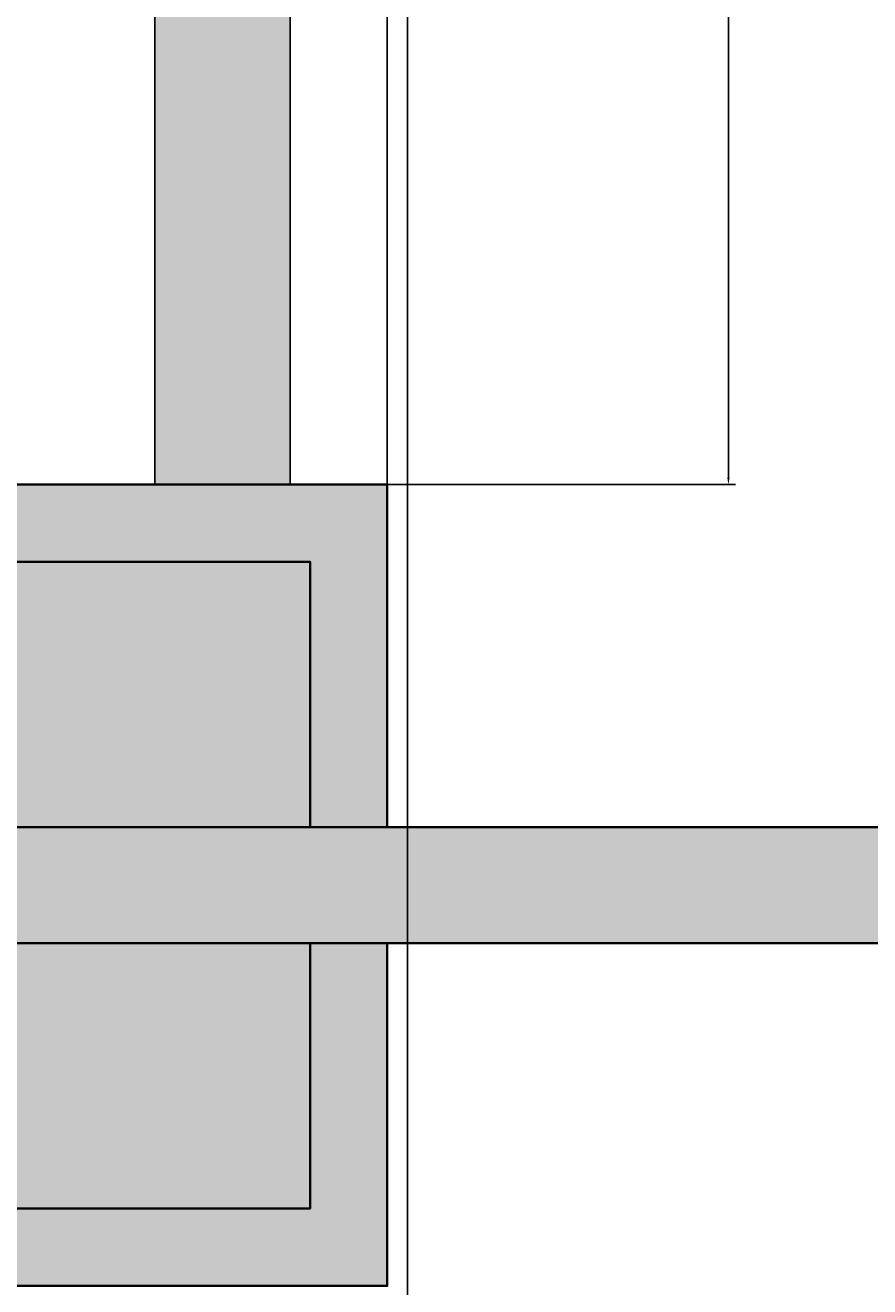
# Model space of a CAD drawing. Units: millimetres. Extents: x -11 to 280, y -4 to 208.
# Tile 36 of 55: x 222 to 244, y 23 to 55. Entities that reach past the tile are written whole.
import ezdxf

# ---------------------------------------------------------------- set-up
doc = ezdxf.new("R2010")
doc.units = ezdxf.units.MM
for name, color, linetype, lineweight in [('M-DIMS', 2, 'Continuous', 18), ('M-HYDR-CYL', 7, 'Continuous', 35), ('M-HYDR-CYL-PATT', 252, 'Continuous', 13), ('M-HYDR-PRES', 7, 'Continuous', 25)]:
    doc.layers.add(name, color=color, linetype=linetype, lineweight=lineweight)
doc.layers.add('M-HYDR-PRES-PATT', color=240, linetype='Continuous', lineweight=13, true_color=0xed1f24)
doc.styles.get("Standard").update_dxf_attribs({"font": 'arial.ttf'})
doc.dimstyles.get("Standard").update_dxf_attribs({"dimtxt": 0.18, "dimasz": 0.18, "dimexe": 0.18, "dimexo": 0.0625, "dimgap": 0.09, "dimtad": 0, "dimtih": 1, "dimtoh": 1, "dimdec": 4, "dimzin": 0, "dimdsep": 46, "dimtxsty": 'Standard', "dimcen": 0.09, "dimadec": 0, "dimazin": 0, "dimtfac": 1, "dimtdec": 4, "dimtofl": 0, "dimtmove": 0, "dimatfit": 3, "dimfxl": 1, "dimtolj": 1, "dimtzin": 0, "dimarcsym": 0})

# ---------------------------------------------------------------- blocks, each defined once
blk = doc.blocks.new('*D4')
at = {"layer": 'Defpoints', "color": 0, "transparency": 16777216}
for p in [(4.763, 84.426), (266.035, 51.733), (266.035, -3.415)]:
    blk.add_point(p, dxfattribs=at)
at = {"layer": 'M-DIMS', "color": 0, "lineweight": -2, "transparency": 16777216}
for p, q in [((4.763, 84.364), (4.763, -3.595)), ((266.035, 51.67), (266.035, -3.595)), ((4.943, -3.415), (134.934, -3.415)), ((265.855, -3.415), (135.864, -3.415))]:
    blk.add_line(p, q, dxfattribs=at)
at = {"layer": 'M-DIMS', "color": 0, "transparency": 16777216}
for points in [[(4.943, -3.385), (4.943, -3.445), (4.763, -3.415)], [(265.855, -3.385), (265.855, -3.445), (266.035, -3.415)]]:
    blk.add_solid(points, dxfattribs=at)
at = {"layer": 'M-DIMS', "color": 0, "transparency": 16777216, "insert": (135.399, -3.415), "char_height": 0.18, "attachment_point": 5}
blk.add_mtext('\\A1;261.27', dxfattribs=at)
blk = doc.blocks.new('*D5')
at = {"layer": 'Defpoints', "color": 0, "transparency": 16777216}
for p in [(24.759, 192.645), (-10.087, 11.435), (261.686, 11.435)]:
    blk.add_point(p, dxfattribs=at)
at = {"layer": 'M-DIMS', "color": 0, "lineweight": -2, "transparency": 16777216}
for p, q in [((24.696, 192.645), (-10.267, 192.645)), ((-10.087, 192.465), (-10.087, 102.222)), ((-10.087, 11.615), (-10.087, 101.858)), ((261.624, 11.435), (-10.267, 11.435))]:
    blk.add_line(p, q, dxfattribs=at)
at = {"layer": 'M-DIMS', "color": 0, "transparency": 16777216}
for points in [[(-10.117, 192.465), (-10.057, 192.465), (-10.087, 192.645)], [(-10.117, 11.615), (-10.057, 11.615), (-10.087, 11.435)]]:
    blk.add_solid(points, dxfattribs=at)
at = {"layer": 'M-DIMS', "color": 0, "transparency": 16777216, "insert": (-10.087, 102.04), "char_height": 0.18, "attachment_point": 5}
blk.add_mtext('\\A1;181.2', dxfattribs=at)
blk = doc.blocks.new('*D13')
at = {"layer": 'Defpoints', "color": 0, "transparency": 16777216}
for p in [(191.774, 105.314), (232.2, 105.314), (232.2, -3.415)]:
    blk.add_point(p, dxfattribs=at)
at = {"layer": 'M-DIMS', "color": 0, "lineweight": -2, "transparency": 16777216}
for p, q in [((191.774, 105.252), (191.774, -3.595)), ((232.2, 105.252), (232.2, -3.595)), ((191.954, -3.415), (211.52, -3.415)), ((232.02, -3.415), (212.454, -3.415))]:
    blk.add_line(p, q, dxfattribs=at)
at = {"layer": 'M-DIMS', "color": 0, "transparency": 16777216}
for points in [[(191.954, -3.385), (191.954, -3.445), (191.774, -3.415)], [(232.02, -3.385), (232.02, -3.445), (232.2, -3.415)]]:
    blk.add_solid(points, dxfattribs=at)
at = {"layer": 'M-DIMS', "color": 0, "transparency": 16777216, "insert": (211.987, -3.415), "char_height": 0.18, "attachment_point": 5}
blk.add_mtext('\\A1;40.426', dxfattribs=at)
blk = doc.blocks.new('*D19')
at = {"layer": 'Defpoints', "color": 0, "transparency": 16777216}
for p in [(225.662, 75.21), (225.662, 43.599), (240.512, 43.599)]:
    blk.add_point(p, dxfattribs=at)
at = {"layer": 'M-DIMS', "color": 0, "lineweight": -2, "transparency": 16777216}
for p, q in [((225.724, 75.21), (240.692, 75.21)), ((240.512, 75.03), (240.512, 59.586)), ((240.512, 43.779), (240.512, 59.222)), ((225.724, 43.599), (240.692, 43.599))]:
    blk.add_line(p, q, dxfattribs=at)
at = {"layer": 'M-DIMS', "color": 0, "transparency": 16777216}
for points in [[(240.482, 75.03), (240.542, 75.03), (240.512, 75.21)], [(240.482, 43.779), (240.542, 43.779), (240.512, 43.599)]]:
    blk.add_solid(points, dxfattribs=at)
at = {"layer": 'M-DIMS', "color": 0, "transparency": 16777216, "insert": (240.512, 59.404), "char_height": 0.18, "attachment_point": 5}
blk.add_mtext('\\A1;31.61', dxfattribs=at)
blk = doc.blocks.new('*D20')
at = {"layer": 'Defpoints', "color": 0, "transparency": 16777216}
for p in [(231.68, 207.495), (151.022, 43.599), (231.68, 43.599)]:
    blk.add_point(p, dxfattribs=at)
at = {"layer": 'M-DIMS', "color": 0, "lineweight": -2, "transparency": 16777216}
for p, q in [((151.022, 43.662), (151.022, 207.675)), ((151.202, 207.495), (190.957, 207.495)), ((231.5, 207.495), (191.745, 207.495)), ((231.68, 43.662), (231.68, 207.675))]:
    blk.add_line(p, q, dxfattribs=at)
at = {"layer": 'M-DIMS', "color": 0, "transparency": 16777216}
for points in [[(151.202, 207.525), (151.202, 207.465), (151.022, 207.495)], [(231.5, 207.525), (231.5, 207.465), (231.68, 207.495)]]:
    blk.add_solid(points, dxfattribs=at)
at = {"layer": 'M-DIMS', "color": 0, "transparency": 16777216, "insert": (191.351, 207.495), "char_height": 0.18, "attachment_point": 5}
blk.add_mtext('\\A1;80.66', dxfattribs=at)
blk = doc.blocks.new('*D22')
at = {"layer": 'Defpoints', "color": 0, "transparency": 16777216}
for p in [(259.871, 207.495), (231.68, 34.723), (259.871, 34.723)]:
    blk.add_point(p, dxfattribs=at)
at = {"layer": 'M-DIMS', "color": 0, "lineweight": -2, "transparency": 16777216}
for p, q in [((231.68, 34.785), (231.68, 207.675)), ((231.86, 207.495), (245.38, 207.495)), ((259.691, 207.495), (246.171, 207.495)), ((259.871, 34.785), (259.871, 207.675))]:
    blk.add_line(p, q, dxfattribs=at)
at = {"layer": 'M-DIMS', "color": 0, "transparency": 16777216}
for points in [[(231.86, 207.525), (231.86, 207.465), (231.68, 207.495)], [(259.691, 207.525), (259.691, 207.465), (259.871, 207.495)]]:
    blk.add_solid(points, dxfattribs=at)
at = {"layer": 'M-DIMS', "color": 0, "transparency": 16777216, "insert": (245.776, 207.495), "char_height": 0.18, "attachment_point": 5}
blk.add_mtext('\\A1;28.19', dxfattribs=at)

msp = doc.modelspace()

# ---------------------------------------------------------------- hatches: boundary and pattern name
at = {"layer": 'M-HYDR-CYL-PATT'}
h = msp.add_hatch(color=256, dxfattribs=at)
h.set_gradient(color1=(128, 128, 128), color2=(99, 100, 102), tint=1)
h.paths.add_polyline_path([(163.0955, 41.5991), (160.6935, 41.5991), (160.6935, 24.846), (163.0955, 24.846)])
h.paths.add_polyline_path([(259.871, 34.7226), (163.0955, 34.7226), (163.0955, 31.7226), (259.871, 31.7226, 1)])
h.paths.add_polyline_path([(257.0171, 42.0966), (265.5958, 50.6754, 1), (263.4745, 52.7967), (253.6316, 42.9537), (253.6316, 34.7226), (257.0171, 34.7226)])
h.paths.add_polyline_path([(257.0171, 25.6028), (257.0171, 31.7226), (253.6316, 31.7226), (253.6316, 26.785), (249.6456, 22.7991), (249.6456, 13.7204, 1), (252.6456, 13.7204), (252.6456, 21.2313)])
h.paths.add_polyline_path([(265.4334, 20.9382), (261.6863, 20.9382), (261.6863, 11.4346), (265.4334, 11.4346)])
h.paths.add_polyline_path([(261.6863, 17.1598), (252.6456, 17.1598), (252.6456, 15.9126), (261.6863, 15.9126)])
h = msp.add_hatch(color=256, dxfattribs=at)
h.set_gradient(color1=(102, 52, 60), color2=(102, 52, 60), tint=1)
h.paths.add_polyline_path([(153.0217, 24.846), (153.0217, 41.5991), (156.2446, 41.5991), (156.2446, 43.5991), (151.0217, 43.5991), (151.0217, 22.846), (231.6803, 22.846), (231.6803, 31.7226), (229.6803, 31.7226), (229.6803, 24.846)])
h.paths.add_polyline_path([(159.7446, 43.5991), (159.7446, 41.5991), (163.0955, 41.5991), (229.6803, 41.5991), (229.6803, 34.7226), (231.6803, 34.7226), (231.6803, 43.5991)], flags=17)
h = msp.add_hatch(color=256, dxfattribs=at)
h.set_gradient(color1=(76, 38, 47), color2=(34, 52, 110), tint=1, name='INVCYLINDER')
h.paths.add_polyline_path([(163.0955, 41.5991), (163.0955, 34.7226), (229.6803, 34.7226), (229.6803, 41.5991)])
h.paths.add_polyline_path([(229.6803, 24.846), (229.6803, 31.7226), (163.0955, 31.7226), (163.0955, 24.846)])
at = {"layer": 'M-HYDR-PRES-PATT'}
h = msp.add_hatch(color=256, dxfattribs=at)
h.set_gradient(color1=(237, 31, 36), color2=(237, 31, 36), tint=1)
h.paths.add_polyline_path([(232.2, 133.1228), (228.7, 133.1228), (228.7, 108.8141), (102.7646, 108.8141), (102.7646, 105.3141), (232.2, 105.3141)])
h.paths.add_polyline_path([(128.8433, 105.3141), (125.3433, 105.3141), (125.3433, 91.7099, 1), (128.8433, 91.7099)])
h.paths.add_polyline_path([(229.1617, 78.7098), (196.7745, 78.7098, -0.4142136), (191.7745, 83.7098), (191.7745, 105.3141), (188.2745, 105.3141), (188.2745, 80.2098, 0.4142136), (193.2745, 75.2098), (225.6617, 75.2098), (225.6617, 43.5991), (229.1617, 43.5991)])
h.paths.add_polyline_path([(102.7646, 110.3704), (95.5776, 110.3704), (95.5776, 103.9022), (102.7646, 103.9022)])
h.paths.add_polyline_path([(100.7059, 107.2502), (99.1711, 106.3641), (99.1711, 106.8641), (97.1711, 106.8641), (97.1711, 107.6363), (99.1711, 107.6363), (99.1711, 108.1363)], flags=16)
h.paths.add_polyline_path([(234.6119, 138.4081), (226.5106, 138.4081), (226.5106, 133.1228), (234.6119, 133.1228)])
h.paths.add_polyline_path([(231.1963, 135.7055), (230.2965, 134.1786), (229.4241, 135.7213), (229.9241, 135.7168), (229.9418, 137.7167), (230.7141, 137.7099), (230.6963, 135.71)], flags=16)

# ---------------------------------------------------------------- linework, layer by layer
at = {"layer": 'M-HYDR-CYL'}
for p, q in [((259.871, 34.7226), (163.0955, 34.7226)), ((259.871, 31.7226), (163.0955, 31.7226))]:
    msp.add_line(p, q, dxfattribs=at)
for points in [[(231.6803, 31.7226), (231.6803, 22.846), (151.0217, 22.846), (151.0217, 43.5991), (156.2446, 43.5991)], [(159.7446, 43.5991), (231.6803, 43.5991), (231.6803, 34.7226)], [(229.6803, 31.7226), (229.6803, 24.846), (153.0217, 24.846), (153.0217, 41.5991), (156.2446, 41.5991)], [(159.7446, 41.5991), (229.6803, 41.5991), (229.6803, 34.7226)]]:
    msp.add_lwpolyline(points, dxfattribs=at)
at = {"layer": 'M-HYDR-PRES'}
for points in [[(188.2745, 105.3141), (188.2745, 80.2098, 0.4142136), (193.2745, 75.2098), (225.6617, 75.2098), (225.6617, 43.5991)], [(191.7745, 105.3141), (191.7745, 83.7098, 0.4142136), (196.7745, 78.7098), (229.1617, 78.7098), (229.1617, 43.5991)]]:
    msp.add_lwpolyline(points, format="xyb", dxfattribs=at)

# ---------------------------------------------------------------- dimensions: what is measured, and where the dimension line sits
at = {"layer": 'M-DIMS'}
for base, p1, p2, override, picture, middle in [((231.6803, 207.495), (151.0217, 43.5991), (231.6803, 43.5991), {"dimdec": 2, "dimlfac": 1, "dimrnd": 0, "dimzin": 0, "dimdsep": 46, "dimlunit": 2}, '*D20', (191.351, 207.495)), ((259.871, 207.495), (231.6803, 34.7226), (259.871, 34.7226), {"dimdec": 2, "dimlfac": 1, "dimrnd": 0, "dimzin": 0, "dimdsep": 46, "dimlunit": 2}, '*D22', (245.7757, 207.495)), ((232.20002, -3.41542), (191.77448, 105.31407), (232.20002, 105.31407), {"dimdec": 3, "dimlfac": 1, "dimrnd": 0, "dimzin": 0, "dimdsep": 46, "dimlunit": 2}, '*D13', (211.98725, -3.41542)), ((266.0352, -3.4154), (4.7635, 84.4261), (266.0352, 51.7328), {"dimdec": 2, "dimlfac": 1, "dimrnd": 0, "dimzin": 0, "dimdsep": 46, "dimlunit": 2}, '*D4', (135.3993, -3.4154))]:
    dim = msp.add_linear_dim(base=base, p1=p1, p2=p2, dimstyle='Standard', override=override, dxfattribs=at)
    dim.commit()
    dim.dimension.update_dxf_attribs({"geometry": picture, "text_midpoint": middle})
for base, p1, p2, angle, override, picture, middle in [((-10.0865, 11.4346), (24.7588, 192.645), (261.6863, 11.4346), 90, {"dimdec": 1, "dimlfac": 1, "dimrnd": 0, "dimzin": 0, "dimdsep": 46, "dimlunit": 2}, '*D5', (-10.0865, 102.0398)), ((240.5117, 43.5991), (225.6617, 75.2098), (225.6617, 43.5991), 270, {"dimdec": 2, "dimlfac": 1, "dimrnd": 0, "dimzin": 0, "dimdsep": 46, "dimlunit": 2}, '*D19', (240.5117, 59.4044))]:
    dim = msp.add_linear_dim(base=base, p1=p1, p2=p2, angle=angle, dimstyle='Standard', override=override, dxfattribs=at)
    dim.commit()
    dim.dimension.update_dxf_attribs({"geometry": picture, "text_midpoint": middle})

doc.saveas('drawing.dxf')
